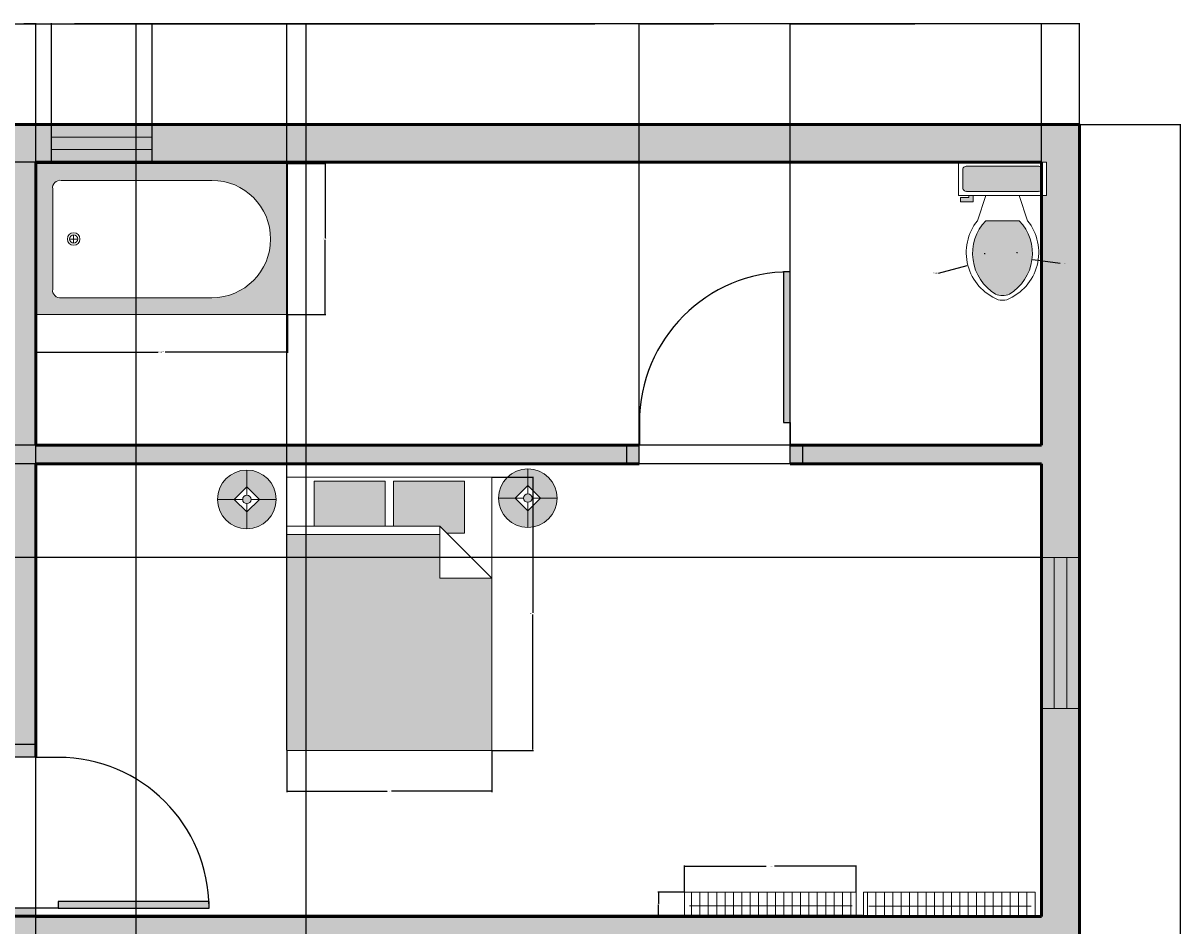
# Model space of a CAD drawing. Units: inches. Extents: x 1201 to 1754, y 247 to 775.
# Tile 10 of 10: x 1475 to 1751, y 560 to 775. Entities that reach past the tile are written whole.
import ezdxf

# ---------------------------------------------------------------- set-up
doc = ezdxf.new("R2010")
doc.units = ezdxf.units.IN
for name, color, linetype, lineweight in [('A-ANNO-DIMS', 2, 'Continuous', 18), ('A-DOOR', 4, 'Continuous', 25), ('A-FLOR-FIXT', 8, 'Continuous', 20), ('A-FLOR-PANL', 8, 'Continuous', 18), ('A-FLOR-PANL-PATT', 8, 'Continuous', 13), ('A-FURN', 8, 'Continuous', 18), ('A-FURN-PATT', 9, 'Continuous', 13), ('A-GLAZ', 4, 'Continuous', 18), ('A-GLAZ-PATT', 9, 'Continuous', 13), ('A-WALL', 7, 'Continuous', 50), ('A-WALL-PATT', 9, 'Continuous', 13)]:
    doc.layers.add(name, color=color, linetype=linetype, lineweight=lineweight)
doc.layers.add('A-DOOR-PATT', color=29, linetype='Continuous', lineweight=13, true_color=0x4f342a)
doc.styles.get("Standard").update_dxf_attribs({"font": 'arial.ttf'})
doc.dimstyles.get("Standard").update_dxf_attribs({"dimtxt": 0.18, "dimasz": 0.18, "dimexe": 0.18, "dimexo": 0.0625, "dimgap": 0.09, "dimtad": 0, "dimtih": 1, "dimtoh": 1, "dimdec": 4, "dimzin": 0, "dimdsep": 46, "dimtxsty": 'Standard', "dimcen": 0.09, "dimadec": 0, "dimazin": 0, "dimtfac": 1, "dimtdec": 4, "dimtofl": 0, "dimtmove": 0, "dimatfit": 3, "dimfxl": 1, "dimtolj": 1, "dimtzin": 0, "dimarcsym": 0})

# ---------------------------------------------------------------- blocks, each defined once
blk = doc.blocks.new('*U2')
for p, q in [((0, 0), (0, -6)), ((-40, 0), (-40, -6))]:
    blk.add_line(p, q)
blk.add_lwpolyline([(0, 0), (0, 40), (-1.75, 40), (-1.75, 0)], close=True)
blk.add_arc((0, 0), 40, 90, 180)
blk = doc.blocks.new('Bed - Queen')
for p, q in [((0, -80.00003), (0, 0)), ((0, 0), (59.99999, 0)), ((59.99999, 0), (59.99999, -80.00003)), ((7.99999, -1.2), (28.79998, -1.2)), ((7.99999, -14.4), (7.99999, -1.2)), ((28.79998, -1.2), (28.79998, -14.4)), ((31.19999, -1.2), (51.99999, -1.2)), ((31.19999, -14.4), (31.19999, -1.2)), ((51.99999, -1.2), (51.99999, -16.4)), ((0, -14.4), (44.8, -14.4)), ((44.8, -16.8), (0, -16.8)), ((59.99999, -29.6), (44.8, -14.4)), ((44.8, -14.4), (44.8, -29.6)), ((51.99999, -16.4), (46.79936, -16.4)), ((44.8, -29.6), (59.99999, -29.6)), ((59.99999, -80.00003), (0, -80.00003))]:
    blk.add_line(p, q)
blk = doc.blocks.new('Lamp - Table')
for p, q in [((0, 7), (0, 1)), ((0, 3), (-3, 0)), ((3, 0), (0, 3)), ((-1, 0), (-7, 0)), ((-3, 0), (0, -3)), ((0, -3), (3, 0)), ((1, 0), (7, 0)), ((0, -1), (0, -7))]:
    blk.add_line(p, q)
for radius in [7, 1]:
    blk.add_circle((0, 0), radius)
blk = doc.blocks.new('Bath Tub - 26 x 60 in.')
for p, q in [((8, -18), (10, -18)), ((9, -17), (9, -19))]:
    blk.add_line(p, q)
blk.add_lwpolyline([(0, -36), (0, 0), (60, 0), (60, -36)], close=True)
for points in [[(6, -4), (42, -4)], [(4, -30), (4, -6)], [(42, -32), (6, -32)]]:
    blk.add_lwpolyline(points)
for radius in [1.5, 1]:
    blk.add_circle((9, -18), radius)
for centre, radius, start, end in [((5.75, -5.75), 1.77, 81.8699, 188.1301), ((42, -18), 14, 270, 90), ((5.75, -30.25), 1.77, 171.8699, 278.1301)]:
    blk.add_arc(centre, radius, start, end)
blk = doc.blocks.new('Toilet - top')
for p, q in [((9.5, -6), (9.5, -2)), ((-8, -8.5), (-8, -8)), ((-7, -8), (-7, -9.5)), ((-4, -8), (-6, -14)), ((4, -8), (6, -14)), ((-10, -8.5), (-8, -8.5)), ((-10, -9.5), (-10, -8.5)), ((-7, -9.5), (-10, -9.5)), ((4, -14), (-4, -14))]:
    blk.add_line(p, q)
blk.add_lwpolyline([(10.5, -8), (10.5, 0), (-10.5, 0), (-10.5, -8)], close=True)
for points in [[(-9.5, -2), (-9.5, -6)], [(8.5, -1), (-8.5, -1)], [(-8.5, -7), (8.5, -7)]]:
    blk.add_lwpolyline(points)
for centre, radius, start, end in [((-8.62, -1.88), 0.884, 81.8699, 188.1301), ((8.62, -1.88), 0.884, 351.8699, 98.1301), ((-8.62, -6.12), 0.884, 171.8699, 278.1301), ((8.62, -6.12), 0.884, 261.8699, 8.1301), ((3.52, -21.58), 12.17, 141.4691, 247.9714), ((4.2, -21.82), 11.33, 136.3677, 238.9468), ((-3.52, -21.58), 12.17, 292.0284, 38.5307), ((-4.2, -21.82), 11.33, 301.053, 43.6321), ((0, -27.88), 4, 245.7318, 294.2682), ((0, -29), 4, 254.8605, 285.1395)]:
    blk.add_arc(centre, radius, start, end)
blk = doc.blocks.new('WIN-36IN-PLAN')
for p, q in [((9, 36), (0, 36)), ((3, 0), (3, 36)), ((6, 0), (6, 36))]:
    blk.add_line(p, q)
blk.add_lwpolyline([(0, 36), (0, 0), (9, 0), (9, 36)])
blk = doc.blocks.new('PANEL-SLATTED-41IN-FRAME')
for p, q in [((40.98, 5.79), (0, 5.79)), ((0, 5.79), (0, 0)), ((40.98, 0), (40.98, 5.79)), ((0, 0), (40.98, 0)), ((40, 2.48), (1.24, 2.48))]:
    blk.add_line(p, q)
blk = doc.blocks.new('*D23')
at = {"layer": 'A-ANNO-DIMS', "color": 0, "lineweight": -2, "transparency": 16777216}
for p, q in [((1586.41, 666.81), (1596.31, 666.81)), ((1596.13, 666.63), (1596.13, 634.38)), ((1596.13, 601.76), (1596.13, 634.01)), ((1586.41, 601.58), (1596.31, 601.58))]:
    blk.add_line(p, q, dxfattribs=at)
at = {"layer": 'A-ANNO-DIMS', "color": 0, "transparency": 16777216}
for points in [[(1596.1, 666.63), (1596.16, 666.63), (1596.13, 666.81)], [(1596.1, 601.76), (1596.16, 601.76), (1596.13, 601.58)]]:
    blk.add_solid(points, dxfattribs=at)
at = {"layer": 'Defpoints', "color": 0, "transparency": 16777216}
for p in [(1586.35, 666.81), (1596.13, 666.81), (1586.35, 601.58)]:
    blk.add_point(p, dxfattribs=at)
at = {"layer": 'A-ANNO-DIMS', "color": 0, "transparency": 16777216, "insert": (1596.13, 634.2), "char_height": 0.18, "attachment_point": 5}
blk.add_mtext('\\A1;BED 65 TYP.', dxfattribs=at)
blk = doc.blocks.new('*D24')
at = {"layer": 'A-ANNO-DIMS', "color": 0, "lineweight": -2, "transparency": 16777216}
for p, q in [((1537.42, 601.52), (1537.42, 591.62)), ((1586.35, 601.52), (1586.35, 591.62)), ((1537.6, 591.8), (1561.35, 591.8)), ((1586.17, 591.8), (1562.42, 591.8))]:
    blk.add_line(p, q, dxfattribs=at)
at = {"layer": 'A-ANNO-DIMS', "color": 0, "transparency": 16777216}
for points in [[(1537.6, 591.83), (1537.6, 591.77), (1537.42, 591.8)], [(1586.17, 591.83), (1586.17, 591.77), (1586.35, 591.8)]]:
    blk.add_solid(points, dxfattribs=at)
at = {"layer": 'Defpoints', "color": 0, "transparency": 16777216}
for p in [(1537.42, 601.58), (1586.35, 601.58), (1586.35, 591.8)]:
    blk.add_point(p, dxfattribs=at)
at = {"layer": 'A-ANNO-DIMS', "color": 0, "transparency": 16777216, "insert": (1561.88, 591.8), "char_height": 0.18, "attachment_point": 5}
blk.add_mtext('\\A1;49 TYP.', dxfattribs=at)
blk = doc.blocks.new('*D25')
at = {"layer": 'A-ANNO-DIMS', "color": 0, "lineweight": -2, "transparency": 16777216}
for p, q in [((1477.57, 705.55), (1477.57, 696.43)), ((1537.57, 705.55), (1537.57, 696.43)), ((1477.75, 696.61), (1506.75, 696.61)), ((1537.39, 696.61), (1508.38, 696.61))]:
    blk.add_line(p, q, dxfattribs=at)
at = {"layer": 'A-ANNO-DIMS', "color": 0, "transparency": 16777216}
for points in [[(1477.75, 696.64), (1477.75, 696.58), (1477.57, 696.61)], [(1537.39, 696.64), (1537.39, 696.58), (1537.57, 696.61)]]:
    blk.add_solid(points, dxfattribs=at)
at = {"layer": 'Defpoints', "color": 0, "transparency": 16777216}
for p in [(1477.57, 705.61), (1537.57, 705.61), (1537.57, 696.61)]:
    blk.add_point(p, dxfattribs=at)
at = {"layer": 'A-ANNO-DIMS', "color": 0, "transparency": 16777216, "insert": (1507.57, 696.61), "char_height": 0.18, "attachment_point": 5}
blk.add_mtext('\\A1;TUB 60 TYP.', dxfattribs=at)
blk = doc.blocks.new('*D26')
at = {"layer": 'A-ANNO-DIMS', "color": 0, "lineweight": -2, "transparency": 16777216}
for p, q in [((1537.63, 741.61), (1546.75, 741.61)), ((1546.57, 741.43), (1546.57, 723.79)), ((1546.57, 705.79), (1546.57, 723.43)), ((1537.63, 705.61), (1546.75, 705.61))]:
    blk.add_line(p, q, dxfattribs=at)
at = {"layer": 'A-ANNO-DIMS', "color": 0, "transparency": 16777216}
for points in [[(1546.54, 741.43), (1546.6, 741.43), (1546.57, 741.61)], [(1546.54, 705.79), (1546.6, 705.79), (1546.57, 705.61)]]:
    blk.add_solid(points, dxfattribs=at)
at = {"layer": 'Defpoints', "color": 0, "transparency": 16777216}
for p in [(1537.57, 741.61), (1546.57, 741.61), (1537.57, 705.61)]:
    blk.add_point(p, dxfattribs=at)
at = {"layer": 'A-ANNO-DIMS', "color": 0, "transparency": 16777216, "insert": (1546.57, 723.61), "char_height": 0.18, "attachment_point": 5}
blk.add_mtext('\\A1;36 TYP.', dxfattribs=at)
blk = doc.blocks.new('*D29')
at = {"layer": 'A-ANNO-DIMS', "color": 0, "lineweight": -2, "transparency": 16777216}
for p, q in [((1632.29, 567.82), (1632.29, 574.09)), ((1632.47, 573.91), (1651.81, 573.91)), ((1673.09, 573.91), (1653.75, 573.91)), ((1673.27, 567.82), (1673.27, 574.09))]:
    blk.add_line(p, q, dxfattribs=at)
at = {"layer": 'A-ANNO-DIMS', "color": 0, "transparency": 16777216}
for points in [[(1632.47, 573.94), (1632.47, 573.88), (1632.29, 573.91)], [(1673.09, 573.94), (1673.09, 573.88), (1673.27, 573.91)]]:
    blk.add_solid(points, dxfattribs=at)
at = {"layer": 'Defpoints', "color": 0, "transparency": 16777216}
for p in [(1673.27, 573.91), (1632.29, 567.76), (1673.27, 567.76)]:
    blk.add_point(p, dxfattribs=at)
at = {"layer": 'A-ANNO-DIMS', "color": 0, "transparency": 16777216, "insert": (1652.78, 573.91), "char_height": 0.18, "attachment_point": 5}
blk.add_mtext('\\A1;PANEL 41 TYP.', dxfattribs=at)
blk = doc.blocks.new('*D30')
at = {"layer": 'A-ANNO-DIMS', "color": 0, "lineweight": -2, "transparency": 16777216}
for p, q in [((1632.22, 567.76), (1625.96, 567.76)), ((1626.14, 567.58), (1626.14, 565.05)), ((1626.14, 562.15), (1626.14, 564.68)), ((1632.22, 561.97), (1625.96, 561.97))]:
    blk.add_line(p, q, dxfattribs=at)
at = {"layer": 'A-ANNO-DIMS', "color": 0, "transparency": 16777216}
for points in [[(1626.11, 567.58), (1626.17, 567.58), (1626.14, 567.76)], [(1626.11, 562.15), (1626.17, 562.15), (1626.14, 561.97)]]:
    blk.add_solid(points, dxfattribs=at)
at = {"layer": 'Defpoints', "color": 0, "transparency": 16777216}
for p in [(1626.14, 567.76), (1632.29, 567.76), (1632.29, 561.97)]:
    blk.add_point(p, dxfattribs=at)
at = {"layer": 'A-ANNO-DIMS', "color": 0, "transparency": 16777216, "insert": (1626.14, 564.87), "char_height": 0.18, "attachment_point": 5}
blk.add_mtext('\\A1;6 TYP.', dxfattribs=at)
blk = doc.blocks.new('*D45')
at = {"layer": 'A-ANNO-DIMS', "color": 0, "lineweight": -2, "transparency": 16777216}
for p, q in [((1246.52, 751), (1246.52, 775.14)), ((1246.7, 774.96), (1486.23, 774.96)), ((1726.34, 774.96), (1486.81, 774.96)), ((1726.52, 751), (1726.52, 775.14))]:
    blk.add_line(p, q, dxfattribs=at)
at = {"layer": 'A-ANNO-DIMS', "color": 0, "transparency": 16777216}
for points in [[(1246.7, 774.99), (1246.7, 774.93), (1246.52, 774.96)], [(1726.34, 774.99), (1726.34, 774.93), (1726.52, 774.96)]]:
    blk.add_solid(points, dxfattribs=at)
at = {"layer": 'Defpoints', "color": 0, "transparency": 16777216}
for p in [(1726.52, 774.96), (1246.52, 750.94), (1726.52, 750.94)]:
    blk.add_point(p, dxfattribs=at)
at = {"layer": 'A-ANNO-DIMS', "color": 0, "transparency": 16777216, "insert": (1486.52, 774.96), "char_height": 0.18, "attachment_point": 5}
blk.add_mtext('\\A1;480', dxfattribs=at)
blk = doc.blocks.new('*D46')
at = {"layer": 'A-ANNO-DIMS', "color": 0, "lineweight": -2, "transparency": 16777216}
for p, q in [((1726.58, 750.94), (1750.72, 750.94)), ((1750.54, 750.76), (1750.54, 511.12)), ((1750.54, 271.12), (1750.54, 510.76)), ((1726.58, 270.94), (1750.72, 270.94))]:
    blk.add_line(p, q, dxfattribs=at)
at = {"layer": 'A-ANNO-DIMS', "color": 0, "transparency": 16777216}
for points in [[(1750.51, 750.76), (1750.57, 750.76), (1750.54, 750.94)], [(1750.51, 271.12), (1750.57, 271.12), (1750.54, 270.94)]]:
    blk.add_solid(points, dxfattribs=at)
at = {"layer": 'Defpoints', "color": 0, "transparency": 16777216}
for p in [(1726.52, 750.94), (1750.54, 750.94), (1726.52, 270.94)]:
    blk.add_point(p, dxfattribs=at)
at = {"layer": 'A-ANNO-DIMS', "color": 0, "transparency": 16777216, "insert": (1750.54, 510.94), "char_height": 0.18, "attachment_point": 5}
blk.add_mtext('\\A1;480', dxfattribs=at)
blk = doc.blocks.new('*D52')
at = {"layer": 'A-ANNO-DIMS', "color": 0, "lineweight": -2, "transparency": 16777216}
for p, q in [((1477.46, 669.94), (1222.33, 669.94)), ((1222.51, 669.76), (1222.51, 616.12)), ((1222.51, 562.12), (1222.51, 615.76)), ((1477.46, 561.94), (1222.33, 561.94))]:
    blk.add_line(p, q, dxfattribs=at)
at = {"layer": 'A-ANNO-DIMS', "color": 0, "transparency": 16777216}
for points in [[(1222.48, 669.76), (1222.54, 669.76), (1222.51, 669.94)], [(1222.48, 562.12), (1222.54, 562.12), (1222.51, 561.94)]]:
    blk.add_solid(points, dxfattribs=at)
at = {"layer": 'Defpoints', "color": 0, "transparency": 16777216}
for p in [(1222.51, 669.94), (1477.52, 669.94), (1477.52, 561.94)]:
    blk.add_point(p, dxfattribs=at)
at = {"layer": 'A-ANNO-DIMS', "color": 0, "transparency": 16777216, "insert": (1222.51, 615.94), "char_height": 0.18, "attachment_point": 5}
blk.add_mtext('\\A1;108', dxfattribs=at)
blk = doc.blocks.new('*D53')
at = {"layer": 'A-ANNO-DIMS', "color": 0, "lineweight": -2, "transparency": 16777216}
for p, q in [((1717.46, 741.94), (1222.33, 741.94)), ((1222.51, 741.76), (1222.51, 708.37)), ((1222.51, 674.62), (1222.51, 708.01)), ((1657.46, 674.44), (1222.33, 674.44))]:
    blk.add_line(p, q, dxfattribs=at)
at = {"layer": 'A-ANNO-DIMS', "color": 0, "transparency": 16777216}
for points in [[(1222.48, 741.76), (1222.54, 741.76), (1222.51, 741.94)], [(1222.48, 674.62), (1222.54, 674.62), (1222.51, 674.44)]]:
    blk.add_solid(points, dxfattribs=at)
at = {"layer": 'Defpoints', "color": 0, "transparency": 16777216}
for p in [(1222.51, 741.94), (1717.52, 741.94), (1657.52, 674.44)]:
    blk.add_point(p, dxfattribs=at)
at = {"layer": 'A-ANNO-DIMS', "color": 0, "transparency": 16777216, "insert": (1222.51, 708.19), "char_height": 0.18, "attachment_point": 5}
blk.add_mtext('\\A1;67.5', dxfattribs=at)
blk = doc.blocks.new('*D55')
at = {"layer": 'A-ANNO-DIMS', "color": 0, "lineweight": -2, "transparency": 16777216}
for p, q in [((1501.52, 418), (1501.52, 775.14)), ((1501.7, 774.96), (1521.44, 774.96)), ((1541.84, 774.96), (1522.1, 774.96)), ((1542.02, 418), (1542.02, 775.14))]:
    blk.add_line(p, q, dxfattribs=at)
at = {"layer": 'A-ANNO-DIMS', "color": 0, "transparency": 16777216}
for points in [[(1501.7, 774.99), (1501.7, 774.93), (1501.52, 774.96)], [(1541.84, 774.99), (1541.84, 774.93), (1542.02, 774.96)]]:
    blk.add_solid(points, dxfattribs=at)
at = {"layer": 'Defpoints', "color": 0, "transparency": 16777216}
for p in [(1542.02, 774.96), (1501.52, 417.94), (1542.02, 417.94)]:
    blk.add_point(p, dxfattribs=at)
at = {"layer": 'A-ANNO-DIMS', "color": 0, "transparency": 16777216, "insert": (1521.77, 774.96), "char_height": 0.18, "attachment_point": 5}
blk.add_mtext('\\A1;40.5', dxfattribs=at)
blk = doc.blocks.new('*D60')
at = {"layer": 'A-ANNO-DIMS', "color": 0, "lineweight": -2, "transparency": 16777216}
for p, q in [((1477.52, 418), (1477.52, 775.14)), ((1477.7, 774.96), (1489.3, 774.96)), ((1501.34, 774.96), (1489.74, 774.96)), ((1501.52, 418), (1501.52, 775.14))]:
    blk.add_line(p, q, dxfattribs=at)
at = {"layer": 'A-ANNO-DIMS', "color": 0, "transparency": 16777216}
for points in [[(1477.7, 774.99), (1477.7, 774.93), (1477.52, 774.96)], [(1501.34, 774.99), (1501.34, 774.93), (1501.52, 774.96)]]:
    blk.add_solid(points, dxfattribs=at)
at = {"layer": 'Defpoints', "color": 0, "transparency": 16777216}
for p in [(1501.52, 774.96), (1477.52, 417.94), (1501.52, 417.94)]:
    blk.add_point(p, dxfattribs=at)
at = {"layer": 'A-ANNO-DIMS', "color": 0, "transparency": 16777216, "insert": (1489.52, 774.96), "char_height": 0.18, "attachment_point": 5}
blk.add_mtext('\\A1;24', dxfattribs=at)
blk = doc.blocks.new('*D66')
at = {"layer": 'A-ANNO-DIMS', "color": 0, "lineweight": -2, "transparency": 16777216}
for p, q in [((1477.52, 674.5), (1477.52, 775.14)), ((1477.7, 774.96), (1549.24, 774.96)), ((1621.34, 774.96), (1549.8, 774.96)), ((1621.52, 674.5), (1621.52, 775.14))]:
    blk.add_line(p, q, dxfattribs=at)
at = {"layer": 'A-ANNO-DIMS', "color": 0, "transparency": 16777216}
for points in [[(1477.7, 774.99), (1477.7, 774.93), (1477.52, 774.96)], [(1621.34, 774.99), (1621.34, 774.93), (1621.52, 774.96)]]:
    blk.add_solid(points, dxfattribs=at)
at = {"layer": 'Defpoints', "color": 0, "transparency": 16777216}
for p in [(1621.52, 774.96), (1477.52, 674.44), (1621.52, 674.44)]:
    blk.add_point(p, dxfattribs=at)
at = {"layer": 'A-ANNO-DIMS', "color": 0, "transparency": 16777216, "insert": (1549.52, 774.96), "char_height": 0.18, "attachment_point": 5}
blk.add_mtext('\\A1;144', dxfattribs=at)
blk = doc.blocks.new('*D67')
at = {"layer": 'A-ANNO-DIMS', "color": 0, "lineweight": -2, "transparency": 16777216}
for p, q in [((1621.52, 674.5), (1621.52, 775.14)), ((1621.7, 774.96), (1639.3, 774.96)), ((1657.34, 774.96), (1639.74, 774.96)), ((1657.52, 674.5), (1657.52, 775.14))]:
    blk.add_line(p, q, dxfattribs=at)
at = {"layer": 'A-ANNO-DIMS', "color": 0, "transparency": 16777216}
for points in [[(1621.7, 774.99), (1621.7, 774.93), (1621.52, 774.96)], [(1657.34, 774.99), (1657.34, 774.93), (1657.52, 774.96)]]:
    blk.add_solid(points, dxfattribs=at)
at = {"layer": 'Defpoints', "color": 0, "transparency": 16777216}
for p in [(1657.52, 774.96), (1621.52, 674.44), (1657.52, 674.44)]:
    blk.add_point(p, dxfattribs=at)
at = {"layer": 'A-ANNO-DIMS', "color": 0, "transparency": 16777216, "insert": (1639.52, 774.96), "char_height": 0.18, "attachment_point": 5}
blk.add_mtext('\\A1;36', dxfattribs=at)
blk = doc.blocks.new('*D68')
at = {"layer": 'A-ANNO-DIMS', "color": 0, "lineweight": -2, "transparency": 16777216}
for p, q in [((1657.52, 674.5), (1657.52, 775.14)), ((1657.7, 774.96), (1687.3, 774.96)), ((1717.34, 774.96), (1687.74, 774.96)), ((1717.52, 674.5), (1717.52, 775.14))]:
    blk.add_line(p, q, dxfattribs=at)
at = {"layer": 'A-ANNO-DIMS', "color": 0, "transparency": 16777216}
for points in [[(1657.7, 774.99), (1657.7, 774.93), (1657.52, 774.96)], [(1717.34, 774.99), (1717.34, 774.93), (1717.52, 774.96)]]:
    blk.add_solid(points, dxfattribs=at)
at = {"layer": 'Defpoints', "color": 0, "transparency": 16777216}
for p in [(1717.52, 774.96), (1657.52, 674.44), (1717.52, 674.44)]:
    blk.add_point(p, dxfattribs=at)
at = {"layer": 'A-ANNO-DIMS', "color": 0, "transparency": 16777216, "insert": (1687.52, 774.96), "char_height": 0.18, "attachment_point": 5}
blk.add_mtext('\\A1;60', dxfattribs=at)
blk = doc.blocks.new('*D76')
at = {"layer": 'A-ANNO-DIMS', "color": 0, "lineweight": -2, "transparency": 16777216}
for p, q in [((1717.46, 669.94), (1222.33, 669.94)), ((1222.51, 669.76), (1222.51, 658.95)), ((1222.51, 647.78), (1222.51, 658.59)), ((1717.46, 647.6), (1222.33, 647.6))]:
    blk.add_line(p, q, dxfattribs=at)
at = {"layer": 'A-ANNO-DIMS', "color": 0, "transparency": 16777216}
for points in [[(1222.48, 669.76), (1222.54, 669.76), (1222.51, 669.94)], [(1222.48, 647.78), (1222.54, 647.78), (1222.51, 647.6)]]:
    blk.add_solid(points, dxfattribs=at)
at = {"layer": 'Defpoints', "color": 0, "transparency": 16777216}
for p in [(1222.51, 669.94), (1717.52, 669.94), (1717.52, 647.6)]:
    blk.add_point(p, dxfattribs=at)
at = {"layer": 'A-ANNO-DIMS', "color": 0, "transparency": 16777216, "insert": (1222.51, 658.77), "char_height": 0.18, "attachment_point": 5}
blk.add_mtext('\\A1;22.34', dxfattribs=at)
blk = doc.blocks.new('*D81')
at = {"layer": 'A-ANNO-DIMS', "color": 0, "lineweight": -2, "transparency": 16777216}
for p, q in [((1505.3, 742), (1505.3, 775.14)), ((1505.48, 774.96), (1610.94, 774.96)), ((1717.34, 774.96), (1611.87, 774.96)), ((1717.52, 742), (1717.52, 775.14))]:
    blk.add_line(p, q, dxfattribs=at)
at = {"layer": 'A-ANNO-DIMS', "color": 0, "transparency": 16777216}
for points in [[(1505.48, 774.99), (1505.48, 774.93), (1505.3, 774.96)], [(1717.34, 774.99), (1717.34, 774.93), (1717.52, 774.96)]]:
    blk.add_solid(points, dxfattribs=at)
at = {"layer": 'Defpoints', "color": 0, "transparency": 16777216}
for p in [(1717.52, 774.96), (1505.3, 741.94), (1717.52, 741.94)]:
    blk.add_point(p, dxfattribs=at)
at = {"layer": 'A-ANNO-DIMS', "color": 0, "transparency": 16777216, "insert": (1611.41, 774.96), "char_height": 0.18, "attachment_point": 5}
blk.add_mtext('\\A1;212.22', dxfattribs=at)
blk = doc.blocks.new('*D82')
at = {"layer": 'A-ANNO-DIMS', "color": 0, "lineweight": -2, "transparency": 16777216}
for p, q in [((1481.3, 742), (1481.3, 775.14)), ((1481.48, 774.96), (1493.08, 774.96)), ((1505.12, 774.96), (1493.52, 774.96)), ((1505.3, 742), (1505.3, 775.14))]:
    blk.add_line(p, q, dxfattribs=at)
at = {"layer": 'A-ANNO-DIMS', "color": 0, "transparency": 16777216}
for points in [[(1481.48, 774.99), (1481.48, 774.93), (1481.3, 774.96)], [(1505.12, 774.99), (1505.12, 774.93), (1505.3, 774.96)]]:
    blk.add_solid(points, dxfattribs=at)
at = {"layer": 'Defpoints', "color": 0, "transparency": 16777216}
for p in [(1505.3, 774.96), (1481.3, 741.94), (1505.3, 741.94)]:
    blk.add_point(p, dxfattribs=at)
at = {"layer": 'A-ANNO-DIMS', "color": 0, "transparency": 16777216, "insert": (1493.3, 774.96), "char_height": 0.18, "attachment_point": 5}
blk.add_mtext('\\A1;24', dxfattribs=at)
blk = doc.blocks.new('*D84')
at = {"layer": 'A-ANNO-DIMS', "color": 0, "lineweight": -2, "transparency": 16777216}
for p, q in [((1471.52, 600), (1471.52, 775.14)), ((1471.7, 774.96), (1474.37, 774.96)), ((1477.34, 774.96), (1474.67, 774.96)), ((1477.52, 600), (1477.52, 775.14))]:
    blk.add_line(p, q, dxfattribs=at)
at = {"layer": 'A-ANNO-DIMS', "color": 0, "transparency": 16777216}
for points in [[(1471.7, 774.99), (1471.7, 774.93), (1471.52, 774.96)], [(1477.34, 774.99), (1477.34, 774.93), (1477.52, 774.96)]]:
    blk.add_solid(points, dxfattribs=at)
at = {"layer": 'Defpoints', "color": 0, "transparency": 16777216}
for p in [(1477.52, 774.96), (1471.52, 599.94), (1477.52, 599.94)]:
    blk.add_point(p, dxfattribs=at)
at = {"layer": 'A-ANNO-DIMS', "color": 0, "transparency": 16777216, "insert": (1474.52, 774.96), "char_height": 0.18, "attachment_point": 5}
blk.add_mtext('\\A1;6', dxfattribs=at)
blk = doc.blocks.new('*D92')
at = {"layer": 'A-ANNO-DIMS', "color": 0, "lineweight": -2, "transparency": 16777216}
for p, q in [((1477.52, 600), (1477.52, 775.14)), ((1477.7, 774.96), (1507.15, 774.96)), ((1537.24, 774.96), (1507.79, 774.96)), ((1537.42, 601.64), (1537.42, 775.14))]:
    blk.add_line(p, q, dxfattribs=at)
at = {"layer": 'A-ANNO-DIMS', "color": 0, "transparency": 16777216}
for points in [[(1477.7, 774.99), (1477.7, 774.93), (1477.52, 774.96)], [(1537.24, 774.99), (1537.24, 774.93), (1537.42, 774.96)]]:
    blk.add_solid(points, dxfattribs=at)
at = {"layer": 'Defpoints', "color": 0, "transparency": 16777216}
for p in [(1537.42, 774.96), (1477.52, 599.94), (1537.42, 601.58)]:
    blk.add_point(p, dxfattribs=at)
at = {"layer": 'A-ANNO-DIMS', "color": 0, "transparency": 16777216, "insert": (1507.47, 774.96), "char_height": 0.18, "attachment_point": 5}
blk.add_mtext('\\A1;59.9', dxfattribs=at)
blk = doc.blocks.new('*D106')
at = {"layer": 'A-ANNO-DIMS', "color": 0, "lineweight": -2, "transparency": 16777216}
for p, q in [((1711.62, 720.41), (1711.8, 720.41)), ((1711.71, 720.32), (1711.71, 720.5)), ((1692.88, 715.47), (1699.76, 717.27))]:
    blk.add_line(p, q, dxfattribs=at)
at = {"layer": 'A-ANNO-DIMS', "color": 0, "transparency": 16777216}
blk.add_solid([(1699.76, 717.3), (1699.77, 717.25), (1699.94, 717.32)], dxfattribs=at)
at = {"layer": 'Defpoints', "color": 0, "transparency": 16777216}
for p in [(1711.71, 720.41), (1699.94, 717.32)]:
    blk.add_point(p, dxfattribs=at)
at = {"layer": 'A-ANNO-DIMS', "color": 0, "transparency": 16777216, "insert": (1692.2, 715.47), "char_height": 0.18, "attachment_point": 5}
blk.add_mtext('\\A1;4X R12.17', dxfattribs=at)
blk = doc.blocks.new('*D107')
at = {"layer": 'A-ANNO-DIMS', "color": 0, "lineweight": -2, "transparency": 16777216}
for p, q in [((1703.9, 720.17), (1704.08, 720.17)), ((1703.99, 720.08), (1703.99, 720.26)), ((1721.95, 717.76), (1715.4, 718.64))]:
    blk.add_line(p, q, dxfattribs=at)
at = {"layer": 'A-ANNO-DIMS', "color": 0, "transparency": 16777216}
blk.add_solid([(1715.4, 718.67), (1715.39, 718.61), (1715.22, 718.66)], dxfattribs=at)
at = {"layer": 'Defpoints', "color": 0, "transparency": 16777216}
for p in [(1703.99, 720.17), (1715.22, 718.66)]:
    blk.add_point(p, dxfattribs=at)
at = {"layer": 'A-ANNO-DIMS', "color": 0, "transparency": 16777216, "insert": (1722.63, 717.76), "char_height": 0.18, "attachment_point": 5}
blk.add_mtext('\\A1;4X R11.33', dxfattribs=at)

msp = doc.modelspace()

# ---------------------------------------------------------------- hatches: boundary and pattern name
at = {"layer": 'A-DOOR-PATT'}
h = msp.add_hatch(color=256, dxfattribs=at)
h.dxf.hatch_style = 1
h.paths.add_polyline_path([(1391.9756, 612.6194), (1390.4026, 612.6194), (1390.4026, 576.699, 0.01094143), (1391.9756, 576.6646)])
h.paths.add_polyline_path([(1471.5208, 621.9415), (1459.5208, 621.9415), (1459.5208, 617.4415), (1471.5208, 617.4415)])
h.paths.add_polyline_path([(1459.4756, 663.2896, 0.01094143), (1457.9026, 663.2551), (1457.9026, 627.3347), (1459.4756, 627.3347)])
h.paths.add_polyline_path([(1477.5208, 602.9415), (1471.5208, 602.9415), (1471.5208, 599.9415), (1477.5208, 599.9415)])
h.paths.add_polyline_path([(1518.8344, 565.5145), (1482.914, 565.5145), (1482.914, 563.9415), (1518.8689, 563.9415, 0.01094143)])
h.paths.add_polyline_path([(1477.5208, 563.9415), (1471.5208, 563.9415), (1471.5208, 561.9692), (1477.5208, 561.9692)])
h.paths.add_polyline_path([(1621.5208, 674.4415), (1618.5208, 674.4415), (1618.5208, 669.9415), (1621.5208, 669.9415)])
h.paths.add_polyline_path([(1660.5208, 674.4415), (1657.5208, 674.4415), (1657.5208, 669.9415), (1660.5208, 669.9415)])
h.paths.add_polyline_path([(1657.509, 715.7896, 0.01094143), (1655.936, 715.7551), (1655.936, 679.8347), (1657.509, 679.8347)])
h.paths.add_polyline_path([(1566.0208, 279.9415), (1563.0208, 279.9415), (1563.0208, 270.9415), (1566.0208, 270.9415)])
h.paths.add_polyline_path([(1567.6389, 321.2551, 0.01094143), (1566.0659, 321.2896), (1566.0659, 285.3347), (1567.6389, 285.3347)])
h.paths.add_polyline_path([(1603.0208, 279.9415), (1602.0208, 279.9415), (1602.0208, 270.9415), (1603.0208, 270.9415)])
h.paths.add_polyline_path([(1641.0208, 279.9415), (1638.0208, 279.9415), (1638.0208, 270.9415), (1641.0208, 270.9415)])
h.paths.add_polyline_path([(1638.0208, 320.3922, 0.01094143), (1636.4477, 320.3578), (1636.4477, 284.4374), (1638.0208, 284.4374)])
at = {"layer": 'A-FLOR-PANL-PATT'}
h = msp.add_hatch(dxfattribs=at)
h.set_pattern_fill('ANSI31', color=256, scale=0.629921, angle=45, style=0)
h.paths.add_polyline_path([(1632.2869, 561.9692), (1673.2701, 561.9692), (1673.2701, 567.7624), (1632.2869, 567.7624)])
h = msp.add_hatch(dxfattribs=at)
h.set_pattern_fill('ANSI31', color=256, scale=0.629921, angle=45, style=0)
h.paths.add_polyline_path([(1675.0242, 561.9415), (1716.0075, 561.9415), (1716.0075, 567.7347), (1675.0242, 567.7347)])
at = {"layer": 'A-FURN-PATT'}
h = msp.add_hatch(color=256, dxfattribs=at)
h.dxf.hatch_style = 1
h.paths.add_polyline_path([(1335.0621, 716.0469), (1322.6678, 716.0469), (1322.6678, 726.4842), (1286.1373, 726.4842), (1286.1373, 674.95), (1335.0621, 674.95)])
h.paths.add_polyline_path([(1328.5388, 739.2047), (1311.5782, 739.2047), (1311.5782, 728.4412), (1322.6678, 728.4412), (1324.2987, 726.8104), (1328.5388, 726.8104)])
h.paths.add_polyline_path([(1309.6212, 739.2047), (1292.6606, 739.2047), (1292.6606, 728.4412), (1309.6212, 728.4412)])
h.paths.add_polyline_path([(1346.7317, 603.3316), (1338.7317, 603.3316, 0.48007965), (1341.0876, 585.8086, 0.21500378), (1344.3757, 585.8086, 0.4800795)])
h.paths.add_polyline_path([(1315.398, 617.4415), (1255.5208, 617.4415), (1255.5208, 581.4415), (1315.398, 581.4415)])
h.paths.add_polyline_path([(1297.398, 585.4415), (1261.398, 585.4415, -0.50000012), (1259.398, 587.4415), (1259.398, 611.4415, -0.50000012), (1261.398, 613.4415), (1297.398, 613.4415, -1)], flags=16)
h.paths.add_polyline_path([(1262.898, 599.4415, -1), (1265.898, 599.4415, -1)], flags=0)
h.paths.add_polyline_path([(1263.398, 599.4415, -1), (1265.398, 599.4415, -1)], flags=0)
h.paths.add_polyline_path([(1352.2316, 615.3316, 0.50000012), (1351.2316, 616.3316), (1334.2316, 616.3316, 0.50000012), (1333.2316, 615.3316), (1333.2316, 611.3316, 0.50000012), (1334.2316, 610.3316), (1351.2316, 610.3316, 0.50000012), (1352.2316, 611.3316)])
h.paths.add_polyline_path([(1335.7316, 609.3316), (1334.7316, 609.3316), (1334.7316, 608.8316), (1332.7316, 608.8316), (1332.7316, 607.8316), (1335.7316, 607.8316)])
h.paths.add_polyline_path([(1537.5652, 741.6115), (1477.5652, 741.6115), (1477.5652, 705.6115), (1537.5652, 705.6115)])
h.paths.add_polyline_path([(1519.5652, 709.6115), (1483.5652, 709.6115, -0.50000012), (1481.5652, 711.6115), (1481.5652, 735.6115, -0.50000012), (1483.5652, 737.6115), (1519.5652, 737.6115, -1)], flags=16)
h.paths.add_polyline_path([(1485.0652, 723.6115, -1), (1488.0652, 723.6115, -1)], flags=0)
h.paths.add_polyline_path([(1485.5652, 723.6115, -1), (1487.5652, 723.6115, -1)], flags=0)
h.paths.add_polyline_path([(1712.1885, 727.9922), (1704.1885, 727.9922, 0.48007965), (1706.5444, 710.4693, 0.21500378), (1709.8325, 710.4693, 0.4800795)])
h.paths.add_polyline_path([(1701.1884, 733.9922), (1700.1884, 733.9922), (1700.1884, 733.4922), (1698.1884, 733.4922), (1698.1884, 732.4922), (1701.1884, 732.4922)])
h.paths.add_polyline_path([(1717.5208, 740.6473, 0.27397494), (1716.6884, 740.9922), (1699.6884, 740.9922, 0.50000012), (1698.6884, 739.9922), (1698.6884, 735.9922, 0.50000012), (1699.6884, 734.9922), (1716.6884, 734.9922, 0.27397494), (1717.5208, 735.3372)])
h.paths.add_polyline_path([(1586.346, 642.6772), (1573.9517, 642.6772), (1573.9517, 653.1145), (1537.4212, 653.1145), (1537.4212, 601.5803), (1586.346, 601.5803)])
h.paths.add_polyline_path([(1579.8227, 665.835), (1562.8621, 665.835), (1562.8621, 655.0715), (1573.9517, 655.0715), (1575.5826, 653.4407), (1579.8227, 653.4407)])
h.paths.add_polyline_path([(1560.9051, 665.835), (1543.9445, 665.835), (1543.9445, 655.0715), (1560.9051, 655.0715)])
h = msp.add_hatch(color=256, dxfattribs=at)
h.dxf.hatch_style = 1
h.paths.add_polyline_path([(1344.212, 734.2435, 1), (1342.212, 734.2435, 1)])
h.paths.add_polyline_path([(1343.212, 741.2435), (1343.212, 737.2435), (1346.212, 734.2435), (1350.212, 734.2435, 0.41421356)])
h.paths.add_polyline_path([(1350.212, 734.2435), (1346.212, 734.2435), (1343.212, 731.2435), (1343.212, 727.2435, 0.41421356)])
h.paths.add_polyline_path([(1343.212, 731.2435), (1340.212, 734.2435), (1336.212, 734.2435, 0.41421356), (1343.212, 727.2435)])
h.paths.add_polyline_path([(1343.212, 737.2435), (1343.212, 741.2435, 0.41421356), (1336.212, 734.2435), (1340.212, 734.2435)])
h.paths.add_polyline_path([(1286.1373, 731.8347), (1286.1373, 734.2435), (1282.5648, 734.2435), (1279.5648, 731.2435), (1279.5648, 727.2435, 0.31468394)])
h.paths.add_polyline_path([(1276.5648, 734.2435), (1272.5648, 734.2435, 0.41421356), (1279.5648, 727.2435), (1279.5648, 731.2435)])
h.paths.add_polyline_path([(1279.5648, 741.2435, 0.41421356), (1272.5648, 734.2435), (1276.5648, 734.2435), (1279.5648, 737.2435)])
h.paths.add_polyline_path([(1286.1373, 736.6524, 0.31468394), (1279.5648, 741.2435), (1279.5648, 737.2435), (1282.5648, 734.2435), (1286.1373, 734.2435)])
h.paths.add_polyline_path([(1278.5648, 734.2435, 1), (1280.5648, 734.2435, 1)])
h.paths.add_polyline_path([(1594.9356, 658.7794), (1591.9356, 661.7794), (1587.9356, 661.7794, 0.41421356), (1594.9356, 654.7794)])
h.paths.add_polyline_path([(1601.9356, 661.7794), (1597.9356, 661.7794), (1594.9356, 658.7794), (1594.9356, 654.7794, 0.41421356)])
h.paths.add_polyline_path([(1594.9356, 668.7794), (1594.9356, 664.7794), (1597.9356, 661.7794), (1601.9356, 661.7794, 0.41421356)])
h.paths.add_polyline_path([(1594.9356, 664.7794), (1594.9356, 668.7794, 0.41421356), (1587.9356, 661.7794), (1591.9356, 661.7794)])
h.paths.add_polyline_path([(1593.9356, 661.7794, 1), (1595.9356, 661.7794, 1)])
h.paths.add_polyline_path([(1528.896, 661.4743, 1), (1526.896, 661.4743, 1)])
h.paths.add_polyline_path([(1527.896, 668.4743), (1527.896, 664.4743), (1530.896, 661.4743), (1534.896, 661.4743, 0.41421356)])
h.paths.add_polyline_path([(1534.896, 661.4743), (1530.896, 661.4743), (1527.896, 658.4743), (1527.896, 654.4743, 0.41421356)])
h.paths.add_polyline_path([(1524.896, 661.4743), (1520.896, 661.4743, 0.41421356), (1527.896, 654.4743), (1527.896, 658.4743)])
h.paths.add_polyline_path([(1527.896, 668.4743, 0.41421356), (1520.896, 661.4743), (1524.896, 661.4743), (1527.896, 664.4743)])
at = {"layer": 'A-GLAZ-PATT'}
h = msp.add_hatch(color=256, dxfattribs=at)
h.dxf.hatch_style = 1
h.set_gradient(color1=(0, 0, 255), color2=(255, 255, 0), name='INVHEMISPHERICAL')
h.paths.add_polyline_path([(1505.2969, 750.9415), (1481.2969, 750.9415), (1481.2969, 747.9415), (1505.2969, 747.9415)])
h.paths.add_polyline_path([(1505.2969, 747.9415), (1481.2969, 747.9415), (1481.2969, 744.9415), (1505.2969, 744.9415)])
h.paths.add_polyline_path([(1505.2969, 744.9415), (1481.2969, 744.9415), (1481.2969, 741.9415), (1505.2969, 741.9415)])
h = msp.add_hatch(color=256, dxfattribs=at)
h.dxf.hatch_style = 1
h.set_gradient(color1=(0, 0, 255), color2=(255, 255, 0), name='INVCYLINDER')
h.paths.add_polyline_path([(1720.5208, 647.6009), (1717.5208, 647.6009), (1717.5208, 611.6009), (1720.5208, 611.6009)])
h.paths.add_polyline_path([(1723.5208, 647.6009), (1720.5208, 647.6009), (1720.5208, 611.6009), (1723.5208, 611.6009)])
h.paths.add_polyline_path([(1726.5208, 647.6009), (1723.5208, 647.6009), (1723.5208, 611.6009), (1726.5208, 611.6009)])
at = {"layer": 'A-WALL-PATT'}
h = msp.add_hatch(color=256, dxfattribs=at)
h.dxf.hatch_style = 1
h.paths.add_polyline_path([(1255.5208, 741.9415), (1471.5208, 741.9415), (1471.5208, 684.2327), (1471.5208, 602.9415), (1477.5208, 602.9415), (1477.5208, 669.9415), (1618.5208, 669.9415), (1618.5208, 674.4415), (1477.5208, 674.4415), (1477.5208, 741.9415), (1481.2969, 741.9415), (1481.2969, 750.9415), (1246.5208, 750.9415), (1246.5208, 700.7954), (1255.5208, 700.7954)])
h.paths.add_polyline_path([(1255.5208, 557.4415), (1399.5208, 557.4415), (1399.5208, 617.4415), (1423.5208, 617.4415), (1423.5208, 621.9415), (1392.0208, 621.9415), (1392.0208, 617.4415), (1395.0208, 617.4415), (1395.0208, 561.9415), (1255.5208, 561.9415), (1255.5208, 571.8878), (1246.5208, 571.8878), (1246.5208, 506.6967), (1255.5208, 506.6967)])
h.paths.add_polyline_path([(1255.5208, 664.7954), (1246.5208, 664.7954), (1246.5208, 595.8878), (1255.398, 595.8878), (1255.398, 617.4415), (1315.398, 617.4415), (1356.0208, 617.4415), (1356.0208, 618.0127), (1356.0208, 621.9415), (1255.5208, 621.9415), (1255.5208, 629.6628)])
h.paths.add_polyline_path([(1255.5208, 470.6967), (1246.5208, 470.6967), (1246.5208, 347.7487), (1255.5208, 347.7487), (1255.5208, 413.4415), (1405.5208, 413.4415), (1405.5208, 417.9415), (1255.5208, 417.9415)])
h.paths.add_polyline_path([(1290.9481, 279.9415), (1255.5208, 279.9415), (1255.5208, 311.7487), (1246.5208, 311.7487), (1246.5208, 270.9415), (1290.9481, 270.9415)])
h.paths.add_polyline_path([(1486.5907, 279.9415), (1477.5208, 279.9415), (1477.5208, 417.9415), (1468.5208, 417.9415), (1468.5208, 413.4415), (1471.5208, 413.4415), (1471.5208, 279.9415), (1399.0105, 279.9415), (1399.0105, 270.9415), (1486.5907, 270.9415)])
h.paths.add_polyline_path([(1563.0208, 279.9415), (1542.0208, 279.9415), (1542.0208, 417.9415), (1501.5208, 417.9415), (1501.5208, 413.4415), (1513.81, 413.4415), (1513.8125, 413.6987), (1537.8114, 413.4623), (1537.5208, 383.9637), (1537.5208, 279.9415), (1522.5907, 279.9415), (1522.5907, 270.9415), (1563.0208, 270.9415)])
h.paths.add_polyline_path([(1726.5208, 404.0342), (1717.5208, 404.0342), (1717.5208, 279.9415), (1641.0208, 279.9415), (1641.0208, 270.9415), (1726.5208, 270.9415)])
h.paths.add_polyline_path([(1726.5208, 507.4363), (1717.5208, 507.4363), (1717.5208, 440.0342), (1726.5208, 440.0342)])
h.paths.add_polyline_path([(1726.5208, 611.6009), (1717.5208, 611.6009), (1717.5208, 561.9415), (1477.5208, 561.9415), (1471.5208, 561.9692), (1471.5208, 557.4415), (1717.5208, 557.4415), (1717.5208, 543.4363), (1726.5208, 543.4363)])
h.paths.add_polyline_path([(1726.5208, 750.9415), (1505.2969, 750.9415), (1505.2969, 741.9415), (1697.6884, 741.9415), (1697.6884, 741.9922), (1718.6884, 741.9922), (1718.6884, 733.9922), (1717.5208, 733.9922), (1717.5208, 674.4415), (1660.5208, 674.4415), (1660.5208, 669.9415), (1717.5208, 669.9415), (1717.5208, 647.6009), (1726.5208, 647.6009)])

# ---------------------------------------------------------------- linework, layer by layer
at = {"layer": 'A-DOOR'}
for p, q in [((1618.5208, 669.9415), (1618.5208, 674.4415)), ((1621.5208, 669.9415), (1621.5208, 674.4415)), ((1657.5208, 669.9415), (1657.5208, 674.4415)), ((1660.5208, 669.9415), (1660.5208, 674.4415)), ((1477.5208, 602.9415), (1471.5208, 602.9415)), ((1477.5208, 599.9415), (1471.5208, 599.9415)), ((1477.5208, 563.9415), (1471.5208, 563.9415)), ((1477.5208, 561.9415), (1477.5208, 563.9415))]:
    msp.add_line(p, q, dxfattribs=at)
at = {"layer": 'A-GLAZ'}
for p, q in [((1505.2969, 747.9415), (1481.2969, 747.9415)), ((1505.2969, 744.9415), (1481.2969, 744.9415))]:
    msp.add_line(p, q, dxfattribs=at)
msp.add_lwpolyline([(1481.2969, 741.9415), (1505.2969, 741.9415), (1505.2969, 750.9415), (1481.2969, 750.9415)], close=True, dxfattribs=at)
at = {"layer": 'A-WALL'}
for p, q in [((1717.5208, 741.9415), (1477.5208, 741.9415)), ((1477.5208, 674.4415), (1477.5208, 741.9415)), ((1717.5208, 674.4415), (1717.5208, 741.9415)), ((1621.5208, 674.4415), (1477.5208, 674.4415)), ((1717.5208, 674.4415), (1657.5208, 674.4415)), ((1477.5208, 599.9415), (1477.5208, 669.9415)), ((1621.5208, 669.9415), (1477.5208, 669.9415)), ((1717.5208, 669.9415), (1657.5208, 669.9415)), ((1717.5208, 561.9415), (1717.5208, 669.9415)), ((1674.7834, 561.9692), (1471.5208, 561.9692)), ((1717.5208, 561.9415), (1477.5208, 561.9415))]:
    msp.add_line(p, q, dxfattribs=at)
msp.add_lwpolyline([(1638.0208, 270.9415), (1726.5208, 270.9415), (1726.5208, 750.9415), (1246.5208, 750.9415), (1246.5208, 270.9415), (1566.0208, 270.9415)], dxfattribs=at)

# ---------------------------------------------------------------- block references
at = {"layer": 'A-DOOR', "xscale": 0.8988714898198789, "yscale": 0.8988714898198789, "zscale": 0.8988714898198789}
msp.add_blockref('*U2', (1657.509, 679.8347), dxfattribs=at)
at = {"layer": 'A-DOOR', "xscale": 0.8988714898198789, "yscale": 0.8988714898198789, "zscale": 0.8988714898198789, "rotation": 270}
msp.add_blockref('*U2', (1482.914, 563.9415), dxfattribs=at)
at = {"layer": 'A-FLOR-FIXT'}
for name, p in [('Bath Tub - 26 x 60 in.', (1477.5652, 741.6115)), ('Toilet - top', (1708.1884, 741.9922))]:
    msp.add_blockref(name, p, dxfattribs=at)
at = {"layer": 'A-FLOR-PANL'}
for p in [(1632.2869, 561.9692), (1675.0242, 561.9415)]:
    msp.add_blockref('PANEL-SLATTED-41IN-FRAME', p, dxfattribs=at)
at = {"layer": 'A-FURN'}
for p in [(1527.896, 661.4743), (1594.9356, 661.7794)]:
    msp.add_blockref('Lamp - Table', p, dxfattribs=at)
at = {"layer": 'A-FURN', "xscale": 0.8154145585976698, "yscale": 0.8154145585976698, "zscale": 0.8154145585976698}
msp.add_blockref('Bed - Queen', (1537.4212, 666.8135), dxfattribs=at)
at = {"layer": 'A-GLAZ'}
msp.add_blockref('WIN-36IN-PLAN', (1717.5208, 611.6009), dxfattribs=at)

# ---------------------------------------------------------------- dimensions: what is measured, and where the dimension line sits
at = {"layer": 'A-ANNO-DIMS'}
for base, p1, p2, override, picture, middle in [((1726.5208, 774.9565), (1246.5208, 750.9415), (1726.5208, 750.9415), {"dimdec": 0, "dimlfac": 1, "dimrnd": 0, "dimzin": 0, "dimdsep": 46, "dimlunit": 2}, '*D45', (1486.5208, 774.9565)), ((1477.5208, 774.9565), (1471.5208, 599.9415), (1477.5208, 599.9415), {"dimdec": 0, "dimlfac": 1, "dimrnd": 0, "dimzin": 0, "dimdsep": 46, "dimlunit": 2}, '*D84', (1474.5208, 774.9565)), ((1501.5208, 774.9565), (1477.5208, 417.9415), (1501.5208, 417.9415), {"dimdec": 0, "dimlfac": 1, "dimrnd": 0, "dimzin": 0, "dimdsep": 46, "dimlunit": 2}, '*D60', (1489.5208, 774.9565)), ((1621.5208, 774.9565), (1477.5208, 674.4415), (1621.5208, 674.4415), {"dimdec": 0, "dimlfac": 1, "dimrnd": 0, "dimzin": 0, "dimdsep": 46, "dimlunit": 2}, '*D66', (1549.5208, 774.9565)), ((1537.4212, 774.9565), (1477.5208, 599.9415), (1537.4212, 601.5803), {"dimdec": 1, "dimlfac": 1, "dimrnd": 0, "dimzin": 0, "dimdsep": 46, "dimlunit": 2}, '*D92', (1507.471, 774.9565)), ((1505.2969, 774.9565), (1481.2969, 741.9415), (1505.2969, 741.9415), {"dimdec": 0, "dimlfac": 1, "dimrnd": 0, "dimzin": 0, "dimdsep": 46, "dimlunit": 2}, '*D82', (1493.2969, 774.9565)), ((1542.0208, 774.9565), (1501.5208, 417.9415), (1542.0208, 417.9415), {"dimdec": 1, "dimlfac": 1, "dimrnd": 0, "dimzin": 0, "dimdsep": 46, "dimlunit": 2}, '*D55', (1521.7708, 774.9565)), ((1717.5208, 774.9565), (1505.2969, 741.9415), (1717.5208, 741.9415), {"dimdec": 2, "dimlfac": 1, "dimrnd": 0, "dimzin": 0, "dimdsep": 46, "dimlunit": 2}, '*D81', (1611.4088, 774.9565)), ((1657.5208, 774.9565), (1621.5208, 674.4415), (1657.5208, 674.4415), {"dimdec": 0, "dimlfac": 1, "dimrnd": 0, "dimzin": 0, "dimdsep": 46, "dimlunit": 2}, '*D67', (1639.5208, 774.9565)), ((1717.5208, 774.9565), (1657.5208, 674.4415), (1717.5208, 674.4415), {"dimdec": 0, "dimlfac": 1, "dimrnd": 0, "dimzin": 0, "dimdsep": 46, "dimlunit": 2}, '*D68', (1687.5208, 774.9565))]:
    dim = msp.add_linear_dim(base=base, p1=p1, p2=p2, dimstyle='Standard', override=override, dxfattribs=at)
    dim.commit()
    dim.dimension.update_dxf_attribs({"geometry": picture, "text_midpoint": middle})
for base, p1, p2, override, picture, middle in [((1750.5358, 750.9415), (1726.5208, 270.9415), (1726.5208, 750.9415), {"dimdec": 0, "dimlfac": 1, "dimrnd": 0, "dimzin": 0, "dimdsep": 46, "dimlunit": 2}, '*D46', (1750.5358, 510.9415)), ((1222.5058, 741.9415), (1657.5208, 674.4415), (1717.5208, 741.9415), {"dimdec": 1, "dimlfac": 1, "dimrnd": 0, "dimzin": 0, "dimdsep": 46, "dimlunit": 2}, '*D53', (1222.5058, 708.1915)), ((1222.5058, 669.9415), (1717.5208, 647.6009), (1717.5208, 669.9415), {"dimdec": 2, "dimlfac": 1, "dimrnd": 0, "dimzin": 0, "dimdsep": 46, "dimlunit": 2}, '*D76', (1222.5058, 658.7712)), ((1222.5058, 669.9415), (1477.5208, 561.9415), (1477.5208, 669.9415), {"dimdec": 0, "dimlfac": 1, "dimrnd": 0, "dimzin": 0, "dimdsep": 46, "dimlunit": 2}, '*D52', (1222.5058, 615.9415))]:
    dim = msp.add_linear_dim(base=base, p1=p1, p2=p2, angle=90, dimstyle='Standard', override=override, dxfattribs=at)
    dim.commit()
    dim.dimension.update_dxf_attribs({"geometry": picture, "text_midpoint": middle})
for base, p1, p2, text, picture, middle in [((1546.5652, 741.6115), (1537.5652, 705.6115), (1537.5652, 741.6115), '<> TYP.', '*D26', (1546.5652, 723.6115)), ((1596.131, 666.8135), (1586.346, 601.5803), (1586.346, 666.8135), 'BED <> TYP.', '*D23', (1596.131, 634.1969)), ((1626.1394, 567.7624), (1632.2869, 561.9692), (1632.2869, 567.7624), '<> TYP.', '*D30', (1626.1394, 564.8658))]:
    dim = msp.add_linear_dim(base=base, p1=p1, p2=p2, angle=90, text=text, dimstyle='Standard', override={"dimdec": 0, "dimlfac": 1, "dimrnd": 0, "dimzin": 0, "dimdsep": 46, "dimlunit": 2}, dxfattribs=at)
    dim.commit()
    dim.dimension.update_dxf_attribs({"geometry": picture, "text_midpoint": middle})
for center, mpoint, picture, middle in [((1711.708, 720.4118), (1699.9382, 717.3201), '*D106', (1692.8764, 715.4651)), ((1703.9885, 720.1749), (1715.2166, 718.6648), '*D107', (1721.9535, 717.7587))]:
    dim = msp.add_radius_dim(center=center, mpoint=mpoint, text='4X <>', dimstyle='Standard', override={"dimdec": 2, "dimlfac": 1, "dimrnd": 0, "dimzin": 0, "dimdsep": 46, "dimlunit": 2}, dxfattribs=at)
    dim.commit()
    dim.dimension.update_dxf_attribs({"geometry": picture, "text_midpoint": middle, "dimtype": 164})
for base, p1, p2, text, picture, middle in [((1537.5652, 696.6115), (1477.5652, 705.6115), (1537.5652, 705.6115), 'TUB <> TYP.', '*D25', (1507.5652, 696.6115)), ((1586.346, 591.7953), (1537.4212, 601.5803), (1586.346, 601.5803), '<> TYP.', '*D24', (1561.8836, 591.7953)), ((1673.2701, 573.9098), (1632.2869, 567.7624), (1673.2701, 567.7624), 'PANEL <> TYP.', '*D29', (1652.7785, 573.9098))]:
    dim = msp.add_linear_dim(base=base, p1=p1, p2=p2, text=text, dimstyle='Standard', override={"dimdec": 0, "dimlfac": 1, "dimrnd": 0, "dimzin": 0, "dimdsep": 46, "dimlunit": 2}, dxfattribs=at)
    dim.commit()
    dim.dimension.update_dxf_attribs({"geometry": picture, "text_midpoint": middle})

doc.saveas('drawing.dxf')
